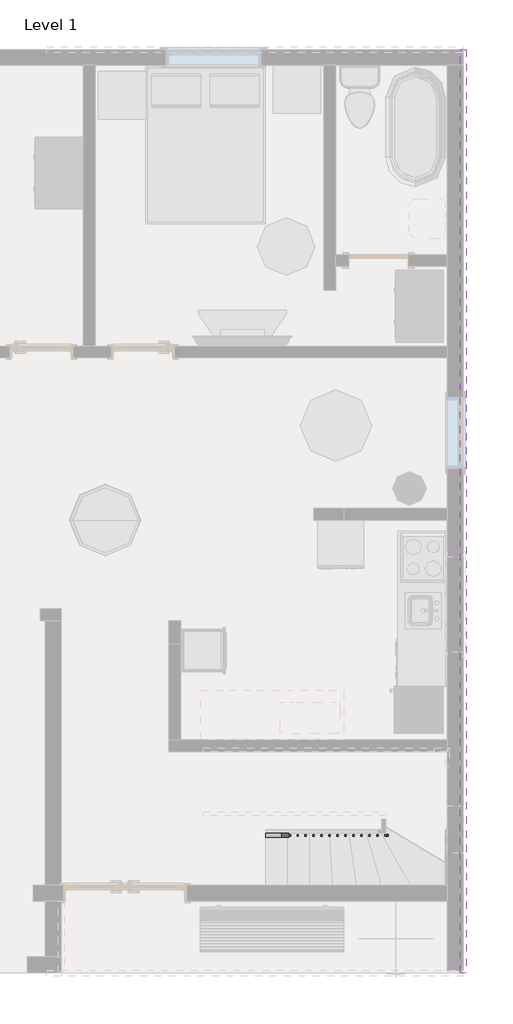
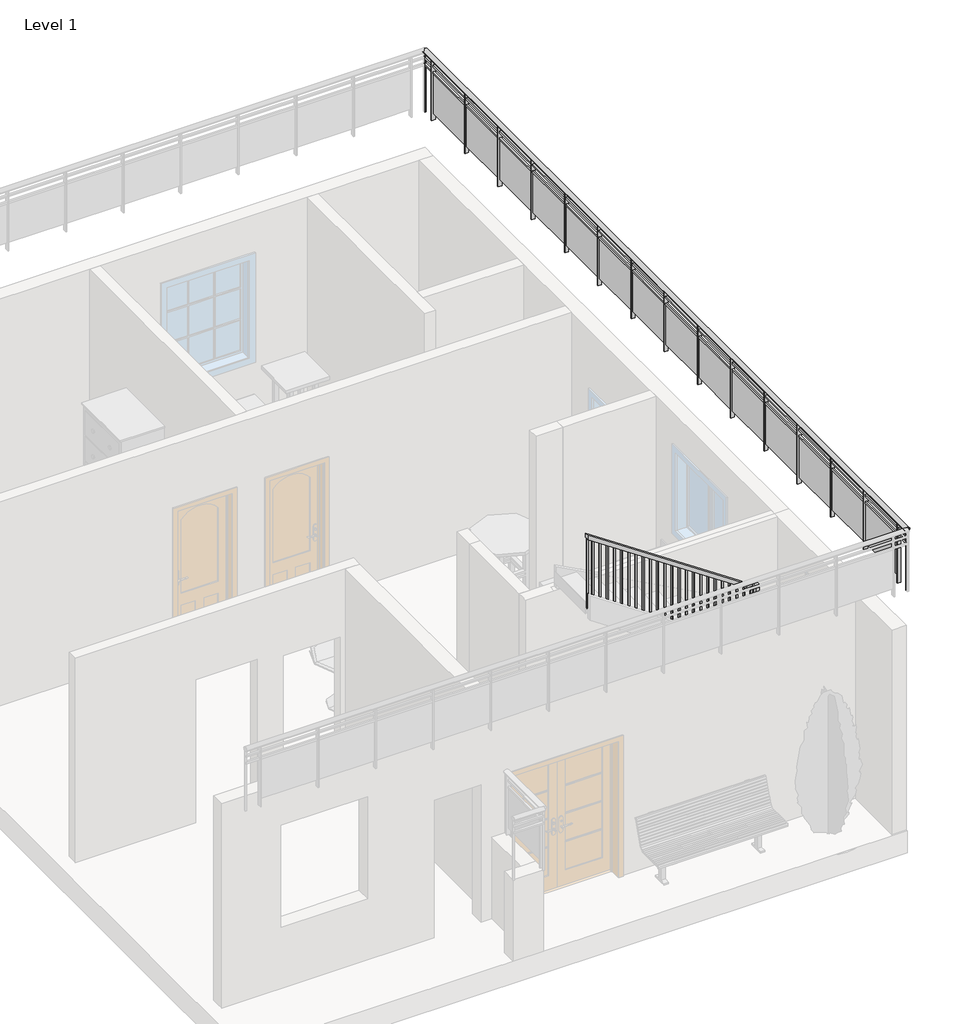
# One storey, part 3 of 4: 2 railings.
"""IFC4 building model written with IfcOpenShell, lengths in millimetres."""

from ifc_helpers import new_model, si_unit, point, frame, origin, place, context, project, spatial, polyline, ellipse_curve, trimmed, outline, extrude, faceted_brep, element, save
from ifc_brep_helpers import plane_surface, extruded_surface, advanced_brep

model = new_model("IFC4")

# Units and contexts
model_context = context("Model", 3, world=origin())
ifc_project = project(units=[si_unit("LENGTHUNIT", "METRE", prefix="MILLI")], contexts=[model_context])

# Site, building, storey
site = spatial("IfcSite", under=ifc_project)
building = spatial("IfcBuilding", under=site)
storey = spatial("IfcBuildingStorey", under=building, Name="Level 1", Elevation=0.0)

# Railings
placement = place(None, origin())
element("IfcRailing", 1, ObjectType="Glass Panel - Bottom Fill", at=placement, inside=storey, context=model_context, shape_type="SolidModel", body=[
    advanced_brep(
    [(5507.3355823, -1680.1159676, 4495.8), (5583.5355823, -1680.1159676, 4495.8), (5507.3355823, 10105.4840324, 4495.8), (5583.5355823, 10105.4840324, 4495.8)],
    [
        (0, 1, ellipse_curve(frame((5545.4355823, -1680.1159676, 4495.8), z_axis=(0.0, -1.0, 0.0), x_axis=(1.0, 0.0, 0.0)), 38.1, 28.575)),
        (1, 0, ellipse_curve(frame((5545.4355823, -1680.1159676, 4495.8), z_axis=(0.0, -1.0, 0.0), x_axis=(1.0, 0.0, 0.0)), 38.1, 28.575)),
        (2, 3, ellipse_curve(frame((5545.4355823, 10105.4840324, 4495.8), z_axis=(0.0, 1.0, 0.0), x_axis=(1.0, 0.0, 0.0)), 38.1, 28.575)),
        (3, 2, ellipse_curve(frame((5545.4355823, 10105.4840324, 4495.8), z_axis=(0.0, 1.0, 0.0), x_axis=(1.0, 0.0, 0.0)), 38.1, 28.575)),
        (0, 2),
        (3, 1),
    ],
    [
        plane_surface(frame((5545.4355823, -1680.1159676, 4495.8), z_axis=(0.0, -1.0, 0.0), x_axis=(0.0, 0.0, 1.0))),
        plane_surface(frame((5545.4355823, 10105.4840324, 4495.8), z_axis=(0.0, 1.0, 0.0), x_axis=(0.0, 0.0, 1.0))),
        extruded_surface(trimmed(ellipse_curve(frame((5545.4355823, 10105.4840324, 4495.8), z_axis=(0.0, -1.0, 0.0), x_axis=(1.0, 0.0, 0.0)), 38.1, 28.575), [point((5507.3355823, 10105.4840324, 4495.8))], [point((5583.5355823, 10105.4840324, 4495.8))], True, "CARTESIAN"), (0.0, -11785.6, 0.0), 11785.6),
        extruded_surface(trimmed(ellipse_curve(frame((5545.4355823, 10105.4840324, 4495.8), z_axis=(0.0, -1.0, 0.0), x_axis=(1.0, 0.0, 0.0)), 38.1, 28.575), [point((5583.5355823, 10105.4840324, 4495.8))], [point((5507.3355823, 10105.4840324, 4495.8))], True, "CARTESIAN"), (0.0, -11785.6, 0.0), 11785.6),
    ],
    [
        (0, [[1, 2]]),
        (1, [[3, 4]]),
        (2, [[-1, 5, -4, 6]]),
        (3, [[-2, -6, -3, -5]]),
    ],
),
    extrude(outline(polyline([(5558.1355823, -1680.1159676), (5532.7355823, -1680.1159676), (5532.7355823, 10105.4840324), (5558.1355823, 10105.4840324), (5558.1355823, -1680.1159676)])), frame((0.0, 0.0, 4381.5), z_axis=(0.0, 0.0, 1.0), x_axis=(1.0, 0.0, 0.0)), (0.0, 0.0, 1.0), 25.4),
    extrude(outline(polyline([(5558.1355823, -1680.1159676), (5532.7355823, -1680.1159676), (5532.7355823, 10105.4840324), (5558.1355823, 10105.4840324), (5558.1355823, -1680.1159676)])), frame((0.0, 0.0, 4279.9), z_axis=(0.0, 0.0, 1.0), x_axis=(1.0, 0.0, 0.0)), (0.0, 0.0, 1.0), 25.4),
    extrude(outline(polyline([(5570.8355823, 9895.9340324), (5520.0355823, 9895.9340324), (5520.0355823, 9908.6340324), (5570.8355823, 9908.6340324), (5570.8355823, 9895.9340324)])), frame((0.0, 0.0, 3581.4), z_axis=(0.0, 0.0, 1.0), x_axis=(1.0, 0.0, 0.0)), (0.0, 0.0, 1.0), 885.6788223),
    extrude(outline(polyline([(5538.9004253, 9089.4840324), (5538.9004253, 9902.2840324), (5545.2504253, 9902.2840324), (5545.2504253, 9089.4840324), (5538.9004253, 9089.4840324)])), frame((0.0, 0.0, 3683.0), z_axis=(0.0, 0.0, 1.0), x_axis=(1.0, 0.0, 0.0)), (0.0, 0.0, 1.0), 596.9),
    extrude(outline(polyline([(5570.8355823, 9083.1340324), (5520.0355823, 9083.1340324), (5520.0355823, 9095.8340324), (5570.8355823, 9095.8340324), (5570.8355823, 9083.1340324)])), frame((0.0, 0.0, 3581.4), z_axis=(0.0, 0.0, 1.0), x_axis=(1.0, 0.0, 0.0)), (0.0, 0.0, 1.0), 885.6788223),
    extrude(outline(polyline([(5538.9004253, 8276.6840324), (5538.9004253, 9089.4840324), (5545.2504253, 9089.4840324), (5545.2504253, 8276.6840324), (5538.9004253, 8276.6840324)])), frame((0.0, 0.0, 3683.0), z_axis=(0.0, 0.0, 1.0), x_axis=(1.0, 0.0, 0.0)), (0.0, 0.0, 1.0), 596.9),
    extrude(outline(polyline([(5570.8355823, 8270.3340324), (5520.0355823, 8270.3340324), (5520.0355823, 8283.0340324), (5570.8355823, 8283.0340324), (5570.8355823, 8270.3340324)])), frame((0.0, 0.0, 3581.4), z_axis=(0.0, 0.0, 1.0), x_axis=(1.0, 0.0, 0.0)), (0.0, 0.0, 1.0), 885.6788223),
    extrude(outline(polyline([(5538.9004253, 7463.8840324), (5538.9004253, 8276.6840324), (5545.2504253, 8276.6840324), (5545.2504253, 7463.8840324), (5538.9004253, 7463.8840324)])), frame((0.0, 0.0, 3683.0), z_axis=(0.0, 0.0, 1.0), x_axis=(1.0, 0.0, 0.0)), (0.0, 0.0, 1.0), 596.9),
    extrude(outline(polyline([(5570.8355823, 7457.5340324), (5520.0355823, 7457.5340324), (5520.0355823, 7470.2340324), (5570.8355823, 7470.2340324), (5570.8355823, 7457.5340324)])), frame((0.0, 0.0, 3581.4), z_axis=(0.0, 0.0, 1.0), x_axis=(1.0, 0.0, 0.0)), (0.0, 0.0, 1.0), 885.6788223),
    extrude(outline(polyline([(5538.9004253, 6651.0840324), (5538.9004253, 7463.8840324), (5545.2504253, 7463.8840324), (5545.2504253, 6651.0840324), (5538.9004253, 6651.0840324)])), frame((0.0, 0.0, 3683.0), z_axis=(0.0, 0.0, 1.0), x_axis=(1.0, 0.0, 0.0)), (0.0, 0.0, 1.0), 596.9),
    extrude(outline(polyline([(5570.8355823, 6644.7340324), (5520.0355823, 6644.7340324), (5520.0355823, 6657.4340324), (5570.8355823, 6657.4340324), (5570.8355823, 6644.7340324)])), frame((0.0, 0.0, 3581.4), z_axis=(0.0, 0.0, 1.0), x_axis=(1.0, 0.0, 0.0)), (0.0, 0.0, 1.0), 885.6788223),
    extrude(outline(polyline([(5538.9004253, 5838.2840324), (5538.9004253, 6651.0840324), (5545.2504253, 6651.0840324), (5545.2504253, 5838.2840324), (5538.9004253, 5838.2840324)])), frame((0.0, 0.0, 3683.0), z_axis=(0.0, 0.0, 1.0), x_axis=(1.0, 0.0, 0.0)), (0.0, 0.0, 1.0), 596.9),
    extrude(outline(polyline([(5570.8355823, 5831.9340324), (5520.0355823, 5831.9340324), (5520.0355823, 5844.6340324), (5570.8355823, 5844.6340324), (5570.8355823, 5831.9340324)])), frame((0.0, 0.0, 3581.4), z_axis=(0.0, 0.0, 1.0), x_axis=(1.0, 0.0, 0.0)), (0.0, 0.0, 1.0), 885.6788223),
    extrude(outline(polyline([(5538.9004253, 5025.4840324), (5538.9004253, 5838.2840324), (5545.2504253, 5838.2840324), (5545.2504253, 5025.4840324), (5538.9004253, 5025.4840324)])), frame((0.0, 0.0, 3683.0), z_axis=(0.0, 0.0, 1.0), x_axis=(1.0, 0.0, 0.0)), (0.0, 0.0, 1.0), 596.9),
    extrude(outline(polyline([(5570.8355823, 5019.1340324), (5520.0355823, 5019.1340324), (5520.0355823, 5031.8340324), (5570.8355823, 5031.8340324), (5570.8355823, 5019.1340324)])), frame((0.0, 0.0, 3581.4), z_axis=(0.0, 0.0, 1.0), x_axis=(1.0, 0.0, 0.0)), (0.0, 0.0, 1.0), 885.6788223),
    extrude(outline(polyline([(5538.9004253, 4212.6840324), (5538.9004253, 5025.4840324), (5545.2504253, 5025.4840324), (5545.2504253, 4212.6840324), (5538.9004253, 4212.6840324)])), frame((0.0, 0.0, 3683.0), z_axis=(0.0, 0.0, 1.0), x_axis=(1.0, 0.0, 0.0)), (0.0, 0.0, 1.0), 596.9),
    extrude(outline(polyline([(5570.8355823, 4206.3340324), (5520.0355823, 4206.3340324), (5520.0355823, 4219.0340324), (5570.8355823, 4219.0340324), (5570.8355823, 4206.3340324)])), frame((0.0, 0.0, 3581.4), z_axis=(0.0, 0.0, 1.0), x_axis=(1.0, 0.0, 0.0)), (0.0, 0.0, 1.0), 885.6788223),
    extrude(outline(polyline([(5538.9004253, 3399.8840324), (5538.9004253, 4212.6840324), (5545.2504253, 4212.6840324), (5545.2504253, 3399.8840324), (5538.9004253, 3399.8840324)])), frame((0.0, 0.0, 3683.0), z_axis=(0.0, 0.0, 1.0), x_axis=(1.0, 0.0, 0.0)), (0.0, 0.0, 1.0), 596.9),
    extrude(outline(polyline([(5570.8355823, 3393.5340324), (5520.0355823, 3393.5340324), (5520.0355823, 3406.2340324), (5570.8355823, 3406.2340324), (5570.8355823, 3393.5340324)])), frame((0.0, 0.0, 3581.4), z_axis=(0.0, 0.0, 1.0), x_axis=(1.0, 0.0, 0.0)), (0.0, 0.0, 1.0), 885.6788223),
    extrude(outline(polyline([(5538.9004253, 2587.0840324), (5538.9004253, 3399.8840324), (5545.2504253, 3399.8840324), (5545.2504253, 2587.0840324), (5538.9004253, 2587.0840324)])), frame((0.0, 0.0, 3683.0), z_axis=(0.0, 0.0, 1.0), x_axis=(1.0, 0.0, 0.0)), (0.0, 0.0, 1.0), 596.9),
    extrude(outline(polyline([(5570.8355823, 2580.7340324), (5520.0355823, 2580.7340324), (5520.0355823, 2593.4340324), (5570.8355823, 2593.4340324), (5570.8355823, 2580.7340324)])), frame((0.0, 0.0, 3581.4), z_axis=(0.0, 0.0, 1.0), x_axis=(1.0, 0.0, 0.0)), (0.0, 0.0, 1.0), 885.6788223),
    extrude(outline(polyline([(5538.9004253, 1774.2840324), (5538.9004253, 2587.0840324), (5545.2504253, 2587.0840324), (5545.2504253, 1774.2840324), (5538.9004253, 1774.2840324)])), frame((0.0, 0.0, 3683.0), z_axis=(0.0, 0.0, 1.0), x_axis=(1.0, 0.0, 0.0)), (0.0, 0.0, 1.0), 596.9),
    extrude(outline(polyline([(5570.8355823, 1767.9340324), (5520.0355823, 1767.9340324), (5520.0355823, 1780.6340324), (5570.8355823, 1780.6340324), (5570.8355823, 1767.9340324)])), frame((0.0, 0.0, 3581.4), z_axis=(0.0, 0.0, 1.0), x_axis=(1.0, 0.0, 0.0)), (0.0, 0.0, 1.0), 885.6788223),
    extrude(outline(polyline([(5538.9004253, 961.4840324), (5538.9004253, 1774.2840324), (5545.2504253, 1774.2840324), (5545.2504253, 961.4840324), (5538.9004253, 961.4840324)])), frame((0.0, 0.0, 3683.0), z_axis=(0.0, 0.0, 1.0), x_axis=(1.0, 0.0, 0.0)), (0.0, 0.0, 1.0), 596.9),
    extrude(outline(polyline([(5570.8355823, 955.1340324), (5520.0355823, 955.1340324), (5520.0355823, 967.8340324), (5570.8355823, 967.8340324), (5570.8355823, 955.1340324)])), frame((0.0, 0.0, 3581.4), z_axis=(0.0, 0.0, 1.0), x_axis=(1.0, 0.0, 0.0)), (0.0, 0.0, 1.0), 885.6788223),
    extrude(outline(polyline([(5538.9004253, 148.6840324), (5538.9004253, 961.4840324), (5545.2504253, 961.4840324), (5545.2504253, 148.6840324), (5538.9004253, 148.6840324)])), frame((0.0, 0.0, 3683.0), z_axis=(0.0, 0.0, 1.0), x_axis=(1.0, 0.0, 0.0)), (0.0, 0.0, 1.0), 596.9),
    extrude(outline(polyline([(5570.8355823, 142.3340324), (5520.0355823, 142.3340324), (5520.0355823, 155.0340324), (5570.8355823, 155.0340324), (5570.8355823, 142.3340324)])), frame((0.0, 0.0, 3581.4), z_axis=(0.0, 0.0, 1.0), x_axis=(1.0, 0.0, 0.0)), (0.0, 0.0, 1.0), 885.6788223),
    extrude(outline(polyline([(5538.9004253, -664.1159676), (5538.9004253, 148.6840324), (5545.2504253, 148.6840324), (5545.2504253, -664.1159676), (5538.9004253, -664.1159676)])), frame((0.0, 0.0, 3683.0), z_axis=(0.0, 0.0, 1.0), x_axis=(1.0, 0.0, 0.0)), (0.0, 0.0, 1.0), 596.9),
    extrude(outline(polyline([(5570.8355823, -670.4659676), (5520.0355823, -670.4659676), (5520.0355823, -657.7659676), (5570.8355823, -657.7659676), (5570.8355823, -670.4659676)])), frame((0.0, 0.0, 3581.4), z_axis=(0.0, 0.0, 1.0), x_axis=(1.0, 0.0, 0.0)), (0.0, 0.0, 1.0), 885.6788223),
    extrude(outline(polyline([(5538.9004253, -1476.9159676), (5538.9004253, -664.1159676), (5545.2504253, -664.1159676), (5545.2504253, -1476.9159676), (5538.9004253, -1476.9159676)])), frame((0.0, 0.0, 3683.0), z_axis=(0.0, 0.0, 1.0), x_axis=(1.0, 0.0, 0.0)), (0.0, 0.0, 1.0), 596.9),
    extrude(outline(polyline([(5570.8355823, -1483.2659676), (5520.0355823, -1483.2659676), (5520.0355823, -1470.5659676), (5570.8355823, -1470.5659676), (5570.8355823, -1483.2659676)])), frame((0.0, 0.0, 3581.4), z_axis=(0.0, 0.0, 1.0), x_axis=(1.0, 0.0, 0.0)), (0.0, 0.0, 1.0), 885.6788223),
    extrude(outline(polyline([(5554.9605823, 10092.7840324), (5535.9105823, 10092.7840324), (5535.9105823, 10111.8340324), (5554.9605823, 10111.8340324), (5554.9605823, 10092.7840324)])), frame((0.0, 0.0, 3581.4), z_axis=(0.0, 0.0, 1.0), x_axis=(1.0, 0.0, 0.0)), (0.0, 0.0, 1.0), 885.6788223),
    extrude(outline(polyline([(5554.9605823, -1686.4659676), (5535.9105823, -1686.4659676), (5535.9105823, -1667.4159676), (5554.9605823, -1667.4159676), (5554.9605823, -1686.4659676)])), frame((0.0, 0.0, 3581.4), z_axis=(0.0, 0.0, 1.0), x_axis=(1.0, 0.0, 0.0)), (0.0, 0.0, 1.0), 885.6788223),
])
element("IfcRailing", 2, ObjectType="Handrail - Rectangular", at=placement, inside=storey, context=model_context, shape_type="SolidModel", body=[
    faceted_brep([(3027.1038904, 97.8840324, 1055.2198174), (3027.1038904, 97.8840324, 992.9732441), (3027.1038904, 47.0840324, 992.9732441), (3027.1038904, 47.0840324, 1055.2198174), (4478.6355823, 97.8840324, 2083.0686785), (4529.4355823, 97.8840324, 2056.7942596), (4529.4355823, 47.0840324, 2056.7942596), (4478.6355823, 47.0840324, 2083.0686785), (4554.8355823, 205.4243752, 2272.2626578), (4554.8355823, 174.0840324, 2323.0626578), (4554.8355823, 301.0840324, 2576.0562227), (4554.8355823, 351.8840324, 2564.0213255), (4605.6355823, 205.4243752, 2272.2626578), (4605.6355823, 351.8840324, 2564.0213255), (4605.6355823, 174.0840324, 2323.0626578), (4605.6355823, 301.0840324, 2576.0562227), (2226.5502663, 377.2840324, 4320.0818974), (2226.5502663, 428.0840324, 4320.0818974), (2226.5502663, 428.0840324, 4258.8171173), (2226.5502663, 377.2840324, 4258.8171173), (4463.1119197, 377.2840324, 2751.11069), (4478.6355823, 377.2840324, 2801.91069), (4463.1119197, 428.0840324, 2751.11069), (4478.6355823, 428.0840324, 2801.91069), (4478.6355823, 97.8840324, 2323.0626578), (4529.4355823, 97.8840324, 2272.2626578), (4529.4355823, 47.0840324, 2272.2626578), (4478.6355823, 47.0840324, 2323.0626578), (4554.8355823, 97.8840324, 2323.0626578), (4554.8355823, 97.8840324, 2272.2626578), (4605.6355823, 47.0840324, 2272.2626578), (4605.6355823, 47.0840324, 2323.0626578), (4554.8355823, 301.0840324, 2801.91069), (4554.8355823, 351.8840324, 2751.11069), (4605.6355823, 351.8840324, 2751.11069), (4605.6355823, 301.0840324, 2801.91069), (4554.8355823, 377.2840324, 2801.91069), (4554.8355823, 377.2840324, 2751.11069), (4605.6355823, 428.0840324, 2751.11069), (4605.6355823, 428.0840324, 2801.91069)], [[[0, 1, 2, 3]], [[1, 0, 4, 5]], [[2, 1, 5, 6]], [[3, 2, 6, 7]], [[0, 3, 7, 4]], [[8, 9, 10, 11]], [[12, 8, 11, 13]], [[14, 12, 13, 15]], [[9, 14, 15, 10]], [[16, 17, 18, 19]], [[20, 21, 16, 19]], [[22, 20, 19, 18]], [[23, 22, 18, 17]], [[21, 23, 17, 16]], [[5, 4, 24, 25]], [[6, 5, 25, 26]], [[7, 6, 26, 27]], [[4, 7, 27, 24]], [[25, 24, 28, 29]], [[26, 25, 29, 30]], [[27, 26, 30, 31]], [[24, 27, 31, 28]], [[29, 28, 9, 8]], [[30, 29, 8, 12]], [[31, 30, 12, 14]], [[28, 31, 14, 9]], [[11, 10, 32, 33]], [[13, 11, 33, 34]], [[15, 13, 34, 35]], [[10, 15, 35, 32]], [[33, 32, 36, 37]], [[34, 33, 37, 38]], [[35, 34, 38, 39]], [[32, 35, 39, 36]], [[37, 36, 21, 20]], [[38, 37, 20, 22]], [[39, 38, 22, 23]], [[36, 39, 23, 21]]]),
    extrude(outline(polyline([(4207.8803949, 2302.1108119), (3217.3333333, 2302.1108119), (3217.3333333, 2321.1608119), (4195.0384473, 2321.1608119), (4207.8803949, 2302.1108119)])), frame((0.0, 393.1590324, 0.0), z_axis=(0.0, 1.0, 0.0), x_axis=(0.0, 0.0, 1.0)), (0.0, 0.0, 1.0), 19.05),
    extrude(outline(polyline([(4139.3900079, 2403.7108119), (3217.3333333, 2403.7108119), (3217.3333333, 2422.7608119), (4126.5480604, 2422.7608119), (4139.3900079, 2403.7108119)])), frame((0.0, 393.1590324, 0.0), z_axis=(0.0, 1.0, 0.0), x_axis=(0.0, 0.0, 1.0)), (0.0, 0.0, 1.0), 19.05),
    extrude(outline(polyline([(4070.899621, 2505.3108119), (3048.0, 2505.3108119), (3048.0, 2524.3608119), (4058.0576735, 2524.3608119), (4070.899621, 2505.3108119)])), frame((0.0, 393.1590324, 0.0), z_axis=(0.0, 1.0, 0.0), x_axis=(0.0, 0.0, 1.0)), (0.0, 0.0, 1.0), 19.05),
    extrude(outline(polyline([(4002.4092341, 2606.9108119), (3048.0, 2606.9108119), (3048.0, 2625.9608119), (3989.5672866, 2625.9608119), (4002.4092341, 2606.9108119)])), frame((0.0, 393.1590324, 0.0), z_axis=(0.0, 1.0, 0.0), x_axis=(0.0, 0.0, 1.0)), (0.0, 0.0, 1.0), 19.05),
    extrude(outline(polyline([(3933.9188472, 2708.5108119), (3048.0, 2708.5108119), (3048.0, 2727.5608119), (3921.0768996, 2727.5608119), (3933.9188472, 2708.5108119)])), frame((0.0, 393.1590324, 0.0), z_axis=(0.0, 1.0, 0.0), x_axis=(0.0, 0.0, 1.0)), (0.0, 0.0, 1.0), 19.05),
    extrude(outline(polyline([(3865.4284603, 2810.1108119), (2878.6666667, 2810.1108119), (2878.6666667, 2829.1608119), (3852.5865127, 2829.1608119), (3865.4284603, 2810.1108119)])), frame((0.0, 393.1590324, 0.0), z_axis=(0.0, 1.0, 0.0), x_axis=(0.0, 0.0, 1.0)), (0.0, 0.0, 1.0), 19.05),
    extrude(outline(polyline([(3796.9380733, 2911.7108119), (2878.6666667, 2911.7108119), (2878.6666667, 2930.7608119), (3784.0961258, 2930.7608119), (3796.9380733, 2911.7108119)])), frame((0.0, 393.1590324, 0.0), z_axis=(0.0, 1.0, 0.0), x_axis=(0.0, 0.0, 1.0)), (0.0, 0.0, 1.0), 19.05),
    extrude(outline(polyline([(3728.4476864, 3013.3108119), (2878.6666667, 3013.3108119), (2878.6666667, 3032.3608119), (3715.6057389, 3032.3608119), (3728.4476864, 3013.3108119)])), frame((0.0, 393.1590324, 0.0), z_axis=(0.0, 1.0, 0.0), x_axis=(0.0, 0.0, 1.0)), (0.0, 0.0, 1.0), 19.05),
    extrude(outline(polyline([(3659.9572995, 3114.9108119), (2709.3333333, 3114.9108119), (2709.3333333, 3133.9608119), (3647.1153519, 3133.9608119), (3659.9572995, 3114.9108119)])), frame((0.0, 393.1590324, 0.0), z_axis=(0.0, 1.0, 0.0), x_axis=(0.0, 0.0, 1.0)), (0.0, 0.0, 1.0), 19.05),
    extrude(outline(polyline([(3591.4669126, 3216.5108119), (2709.3333333, 3216.5108119), (2709.3333333, 3235.5608119), (3578.624965, 3235.5608119), (3591.4669126, 3216.5108119)])), frame((0.0, 393.1590324, 0.0), z_axis=(0.0, 1.0, 0.0), x_axis=(0.0, 0.0, 1.0)), (0.0, 0.0, 1.0), 19.05),
    extrude(outline(polyline([(3522.9765256, 3318.1108119), (2540.0, 3318.1108119), (2540.0, 3337.1608119), (3510.1345781, 3337.1608119), (3522.9765256, 3318.1108119)])), frame((0.0, 393.1590324, 0.0), z_axis=(0.0, 1.0, 0.0), x_axis=(0.0, 0.0, 1.0)), (0.0, 0.0, 1.0), 19.05),
    extrude(outline(polyline([(3454.4861387, 3419.7108119), (2540.0, 3419.7108119), (2540.0, 3438.7608119), (3441.6441912, 3438.7608119), (3454.4861387, 3419.7108119)])), frame((0.0, 393.1590324, 0.0), z_axis=(0.0, 1.0, 0.0), x_axis=(0.0, 0.0, 1.0)), (0.0, 0.0, 1.0), 19.05),
    extrude(outline(polyline([(3385.9957518, 3521.3108119), (2540.0, 3521.3108119), (2540.0, 3540.3608119), (3373.1538043, 3540.3608119), (3385.9957518, 3521.3108119)])), frame((0.0, 393.1590324, 0.0), z_axis=(0.0, 1.0, 0.0), x_axis=(0.0, 0.0, 1.0)), (0.0, 0.0, 1.0), 19.05),
    extrude(outline(polyline([(3317.5053649, 3622.9108119), (2370.6666667, 3622.9108119), (2370.6666667, 3641.9608119), (3304.6634173, 3641.9608119), (3317.5053649, 3622.9108119)])), frame((0.0, 393.1590324, 0.0), z_axis=(0.0, 1.0, 0.0), x_axis=(0.0, 0.0, 1.0)), (0.0, 0.0, 1.0), 19.05),
    extrude(outline(polyline([(3249.014978, 3724.5108119), (2370.6666667, 3724.5108119), (2370.6666667, 3743.5608119), (3236.1730304, 3743.5608119), (3249.014978, 3724.5108119)])), frame((0.0, 393.1590324, 0.0), z_axis=(0.0, 1.0, 0.0), x_axis=(0.0, 0.0, 1.0)), (0.0, 0.0, 1.0), 19.05),
    extrude(outline(polyline([(3180.524591, 3826.1108119), (2370.6666667, 3826.1108119), (2370.6666667, 3845.1608119), (3167.6826435, 3845.1608119), (3180.524591, 3826.1108119)])), frame((0.0, 393.1590324, 0.0), z_axis=(0.0, 1.0, 0.0), x_axis=(0.0, 0.0, 1.0)), (0.0, 0.0, 1.0), 19.05),
    extrude(outline(polyline([(3112.0342041, 3927.7108119), (2201.3333333, 3927.7108119), (2201.3333333, 3946.7608119), (3099.1922566, 3946.7608119), (3112.0342041, 3927.7108119)])), frame((0.0, 393.1590324, 0.0), z_axis=(0.0, 1.0, 0.0), x_axis=(0.0, 0.0, 1.0)), (0.0, 0.0, 1.0), 19.05),
    extrude(outline(polyline([(3043.5438172, 4029.3108119), (2201.3333333, 4029.3108119), (2201.3333333, 4048.3608119), (3030.7018697, 4048.3608119), (3043.5438172, 4029.3108119)])), frame((0.0, 393.1590324, 0.0), z_axis=(0.0, 1.0, 0.0), x_axis=(0.0, 0.0, 1.0)), (0.0, 0.0, 1.0), 19.05),
    extrude(outline(polyline([(2975.0534303, 4130.9108119), (2032.0, 4130.9108119), (2032.0, 4149.9608119), (2962.2114827, 4149.9608119), (2975.0534303, 4130.9108119)])), frame((0.0, 393.1590324, 0.0), z_axis=(0.0, 1.0, 0.0), x_axis=(0.0, 0.0, 1.0)), (0.0, 0.0, 1.0), 19.05),
    extrude(outline(polyline([(2906.5630434, 4232.5108119), (2032.0, 4232.5108119), (2032.0, 4251.5608119), (2893.7210958, 4251.5608119), (2906.5630434, 4232.5108119)])), frame((0.0, 393.1590324, 0.0), z_axis=(0.0, 1.0, 0.0), x_axis=(0.0, 0.0, 1.0)), (0.0, 0.0, 1.0), 19.05),
    extrude(outline(polyline([(2838.0726564, 4334.1108119), (1862.6666667, 4334.1108119), (1862.6666667, 4353.1608119), (2825.2307089, 4353.1608119), (2838.0726564, 4334.1108119)])), frame((0.0, 393.1590324, 0.0), z_axis=(0.0, 1.0, 0.0), x_axis=(0.0, 0.0, 1.0)), (0.0, 0.0, 1.0), 19.05),
    extrude(outline(polyline([(2769.5822695, 4435.7108119), (1862.6666667, 4435.7108119), (1862.6666667, 4454.7608119), (2756.740322, 4454.7608119), (2769.5822695, 4435.7108119)])), frame((0.0, 393.1590324, 0.0), z_axis=(0.0, 1.0, 0.0), x_axis=(0.0, 0.0, 1.0)), (0.0, 0.0, 1.0), 19.05),
    extrude(outline(polyline([(4570.7105823, 376.379485), (4570.7105823, 395.429485), (4589.7605823, 395.429485), (4589.7605823, 376.379485), (4570.7105823, 376.379485)])), frame((0.0, 0.0, 1693.3333333), z_axis=(0.0, 0.0, 1.0), x_axis=(1.0, 0.0, 0.0)), (0.0, 0.0, 1.0), 1057.7773567),
    extrude(outline(polyline([(293.829485, 2448.3722946), (293.829485, 1524.0), (274.779485, 1524.0), (274.779485, 2410.4232599), (293.829485, 2448.3722946)])), frame((4570.7105823, 0.0, 0.0), z_axis=(1.0, 0.0, 0.0), x_axis=(0.0, 1.0, 0.0)), (0.0, 0.0, 1.0), 19.05),
    extrude(outline(polyline([(192.229485, 2245.9774427), (192.229485, 1354.6666667), (173.179485, 1354.6666667), (173.179485, 2208.0284079), (192.229485, 2245.9774427)])), frame((4570.7105823, 0.0, 0.0), z_axis=(1.0, 0.0, 0.0), x_axis=(0.0, 1.0, 0.0)), (0.0, 0.0, 1.0), 19.05),
    extrude(outline(polyline([(4541.5788904, 82.0090324), (4560.6288904, 82.0090324), (4560.6288904, 62.9590324), (4541.5788904, 62.9590324), (4541.5788904, 82.0090324)])), frame((0.0, 0.0, 1185.3333333), z_axis=(0.0, 0.0, 1.0), x_axis=(1.0, 0.0, 0.0)), (0.0, 0.0, 1.0), 1086.9293245),
    extrude(outline(polyline([(1993.4487885, 4439.9788904), (1016.0, 4439.9788904), (1016.0, 4459.0288904), (2006.9383464, 4459.0288904), (1993.4487885, 4439.9788904)])), frame((0.0, 62.9590324, 0.0), z_axis=(0.0, 1.0, 0.0), x_axis=(0.0, 0.0, 1.0)), (0.0, 0.0, 1.0), 19.05),
    extrude(outline(polyline([(1921.5044797, 4338.3788904), (1016.0, 4338.3788904), (1016.0, 4357.4288904), (1934.9940376, 4357.4288904), (1921.5044797, 4338.3788904)])), frame((0.0, 62.9590324, 0.0), z_axis=(0.0, 1.0, 0.0), x_axis=(0.0, 0.0, 1.0)), (0.0, 0.0, 1.0), 19.05),
    extrude(outline(polyline([(1849.5601708, 4236.7788904), (846.6666667, 4236.7788904), (846.6666667, 4255.8288904), (1863.0497287, 4255.8288904), (1849.5601708, 4236.7788904)])), frame((0.0, 62.9590324, 0.0), z_axis=(0.0, 1.0, 0.0), x_axis=(0.0, 0.0, 1.0)), (0.0, 0.0, 1.0), 19.05),
    extrude(outline(polyline([(1777.615862, 4135.1788904), (846.6666667, 4135.1788904), (846.6666667, 4154.2288904), (1791.1054199, 4154.2288904), (1777.615862, 4135.1788904)])), frame((0.0, 62.9590324, 0.0), z_axis=(0.0, 1.0, 0.0), x_axis=(0.0, 0.0, 1.0)), (0.0, 0.0, 1.0), 19.05),
    extrude(outline(polyline([(1705.6715532, 4033.5788904), (677.3333333, 4033.5788904), (677.3333333, 4052.6288904), (1719.1611111, 4052.6288904), (1705.6715532, 4033.5788904)])), frame((0.0, 62.9590324, 0.0), z_axis=(0.0, 1.0, 0.0), x_axis=(0.0, 0.0, 1.0)), (0.0, 0.0, 1.0), 19.05),
    extrude(outline(polyline([(1633.7272444, 3931.9788904), (677.3333333, 3931.9788904), (677.3333333, 3951.0288904), (1647.2168023, 3951.0288904), (1633.7272444, 3931.9788904)])), frame((0.0, 62.9590324, 0.0), z_axis=(0.0, 1.0, 0.0), x_axis=(0.0, 0.0, 1.0)), (0.0, 0.0, 1.0), 19.05),
    extrude(outline(polyline([(1561.7829356, 3830.3788904), (508.0, 3830.3788904), (508.0, 3849.4288904), (1575.2724935, 3849.4288904), (1561.7829356, 3830.3788904)])), frame((0.0, 62.9590324, 0.0), z_axis=(0.0, 1.0, 0.0), x_axis=(0.0, 0.0, 1.0)), (0.0, 0.0, 1.0), 19.05),
    extrude(outline(polyline([(1489.8386268, 3728.7788904), (508.0, 3728.7788904), (508.0, 3747.8288904), (1503.3281847, 3747.8288904), (1489.8386268, 3728.7788904)])), frame((0.0, 62.9590324, 0.0), z_axis=(0.0, 1.0, 0.0), x_axis=(0.0, 0.0, 1.0)), (0.0, 0.0, 1.0), 19.05),
    extrude(outline(polyline([(1417.894318, 3627.1788904), (508.0, 3627.1788904), (508.0, 3646.2288904), (1431.3838759, 3646.2288904), (1417.894318, 3627.1788904)])), frame((0.0, 62.9590324, 0.0), z_axis=(0.0, 1.0, 0.0), x_axis=(0.0, 0.0, 1.0)), (0.0, 0.0, 1.0), 19.05),
    extrude(outline(polyline([(1345.9500092, 3525.5788904), (338.6666667, 3525.5788904), (338.6666667, 3544.6288904), (1359.4395671, 3544.6288904), (1345.9500092, 3525.5788904)])), frame((0.0, 62.9590324, 0.0), z_axis=(0.0, 1.0, 0.0), x_axis=(0.0, 0.0, 1.0)), (0.0, 0.0, 1.0), 19.05),
    extrude(outline(polyline([(1274.0057004, 3423.9788904), (338.6666667, 3423.9788904), (338.6666667, 3443.0288904), (1287.4952583, 3443.0288904), (1274.0057004, 3423.9788904)])), frame((0.0, 62.9590324, 0.0), z_axis=(0.0, 1.0, 0.0), x_axis=(0.0, 0.0, 1.0)), (0.0, 0.0, 1.0), 19.05),
    extrude(outline(polyline([(1202.0613916, 3322.3788904), (338.6666667, 3322.3788904), (338.6666667, 3341.4288904), (1215.5509495, 3341.4288904), (1202.0613916, 3322.3788904)])), frame((0.0, 62.9590324, 0.0), z_axis=(0.0, 1.0, 0.0), x_axis=(0.0, 0.0, 1.0)), (0.0, 0.0, 1.0), 19.05),
    extrude(outline(polyline([(1130.1170828, 3220.7788904), (169.3333333, 3220.7788904), (169.3333333, 3239.8288904), (1143.6066407, 3239.8288904), (1130.1170828, 3220.7788904)])), frame((0.0, 62.9590324, 0.0), z_axis=(0.0, 1.0, 0.0), x_axis=(0.0, 0.0, 1.0)), (0.0, 0.0, 1.0), 19.05),
    extrude(outline(polyline([(1058.172774, 3119.1788904), (169.3333333, 3119.1788904), (169.3333333, 3138.2288904), (1071.6623319, 3138.2288904), (1058.172774, 3119.1788904)])), frame((0.0, 62.9590324, 0.0), z_axis=(0.0, 1.0, 0.0), x_axis=(0.0, 0.0, 1.0)), (0.0, 0.0, 1.0), 19.05),
    extrude(outline(polyline([(4556.3608119, 393.1590324), (4537.3108119, 393.1590324), (4537.3108119, 412.2090324), (4556.3608119, 412.2090324), (4556.3608119, 393.1590324)])), frame((0.0, 0.0, 1693.3333333), z_axis=(0.0, 0.0, 1.0), x_axis=(1.0, 0.0, 0.0)), (0.0, 0.0, 1.0), 1057.7773567),
    extrude(outline(polyline([(4570.7105823, 393.1590324), (4570.7105823, 412.2090324), (4589.7605823, 412.2090324), (4589.7605823, 393.1590324), (4570.7105823, 393.1590324)])), frame((0.0, 0.0, 1693.3333333), z_axis=(0.0, 0.0, 1.0), x_axis=(1.0, 0.0, 0.0)), (0.0, 0.0, 1.0), 1057.7773567),
    extrude(outline(polyline([(4570.7105823, 381.8565553), (4570.7105823, 400.9065553), (4589.7605823, 400.9065553), (4589.7605823, 381.8565553), (4570.7105823, 381.8565553)])), frame((0.0, 0.0, 1693.3333333), z_axis=(0.0, 0.0, 1.0), x_axis=(1.0, 0.0, 0.0)), (0.0, 0.0, 1.0), 1057.7773567),
    extrude(outline(polyline([(4570.7105823, 71.579485), (4570.7105823, 90.629485), (4589.7605823, 90.629485), (4589.7605823, 71.579485), (4570.7105823, 71.579485)])), frame((0.0, 0.0, 1185.3333333), z_axis=(0.0, 0.0, 1.0), x_axis=(1.0, 0.0, 0.0)), (0.0, 0.0, 1.0), 1086.9293245),
    extrude(outline(polyline([(4570.7105823, 82.0090324), (4589.7605823, 82.0090324), (4589.7605823, 62.9590324), (4570.7105823, 62.9590324), (4570.7105823, 82.0090324)])), frame((0.0, 0.0, 1185.3333333), z_axis=(0.0, 0.0, 1.0), x_axis=(1.0, 0.0, 0.0)), (0.0, 0.0, 1.0), 1086.9293245),
    extrude(outline(polyline([(4546.4593907, 82.0090324), (4565.5093907, 82.0090324), (4565.5093907, 62.9590324), (4546.4593907, 62.9590324), (4546.4593907, 82.0090324)])), frame((0.0, 0.0, 1185.3333333), z_axis=(0.0, 0.0, 1.0), x_axis=(1.0, 0.0, 0.0)), (0.0, 0.0, 1.0), 1086.9293245),
    extrude(outline(polyline([(4258.8171173, 2226.5502663), (3217.3333333, 2226.5502663), (3217.3333333, 2245.6002663), (4245.9751698, 2245.6002663), (4258.8171173, 2226.5502663)])), frame((0.0, 393.1590324, 0.0), z_axis=(0.0, 1.0, 0.0), x_axis=(0.0, 0.0, 1.0)), (0.0, 0.0, 1.0), 19.05),
    extrude(outline(polyline([(992.9732441, 3027.1038904), (169.3333333, 3027.1038904), (169.3333333, 3046.1538904), (1006.462802, 3046.1538904), (992.9732441, 3027.1038904)])), frame((0.0, 62.9590324, 0.0), z_axis=(0.0, 1.0, 0.0), x_axis=(0.0, 0.0, 1.0)), (0.0, 0.0, 1.0), 19.05),
])

save(model, "model.ifc")

# Revit data of these elements
# Type "Glass Panel - Bottom Fill"
#   Assembly Code = "C2010400"
#   built-in parameter 1008612 = 0.0416667 (stored number, unit not read)
#   built-in parameter 1008611 = 0.0416667 (stored number, unit not read)
#   built-in parameter 1008609 = 0.333333 (stored number, unit not read)
#   built-in parameter 1008604 = 0.166667 (stored number, unit not read)
#   built-in parameter 1008603 = 0.166667 (stored number, unit not read)
#   Railing Height = 3' - 0"
#   built-in parameter 1008630 = 2
#   built-in parameter 1008610 = 2
#   built-in parameter 1008618 = Baluster - Square : 3/4"
# Type "Handrail - Rectangular"
#   Assembly Code = "C2010400"
#   built-in parameter 1008612 = 0.0416667 (stored number, unit not read)
#   built-in parameter 1008611 = 0.0416667 (stored number, unit not read)
#   built-in parameter 1008609 = 0.333333 (stored number, unit not read)
#   built-in parameter 1008604 = 0.166667 (stored number, unit not read)
#   built-in parameter 1008603 = 0.166667 (stored number, unit not read)
#   Railing Height = 3' - 0"
#   built-in parameter 1008630 = 2
#   built-in parameter 1008610 = 2
#   built-in parameter 1008618 = Baluster - Square : 3/4"
# Element 1 (IfcRailing, "Glass Panel - Bottom Fill")
#   built-in parameter 1008621 = 11.75 (stored number, unit not read)
#   Phase Created = New Construction
#   Materials on its faces: "Glass"
# Element 2 (IfcRailing, "Handrail - Rectangular")
#   Phase Created = New Construction
# Materials
#   "Glass": class "Glass", colour RGB 0 128 192, transparency 0.75, Description = "Soda Lime Glass", Cost = 0
